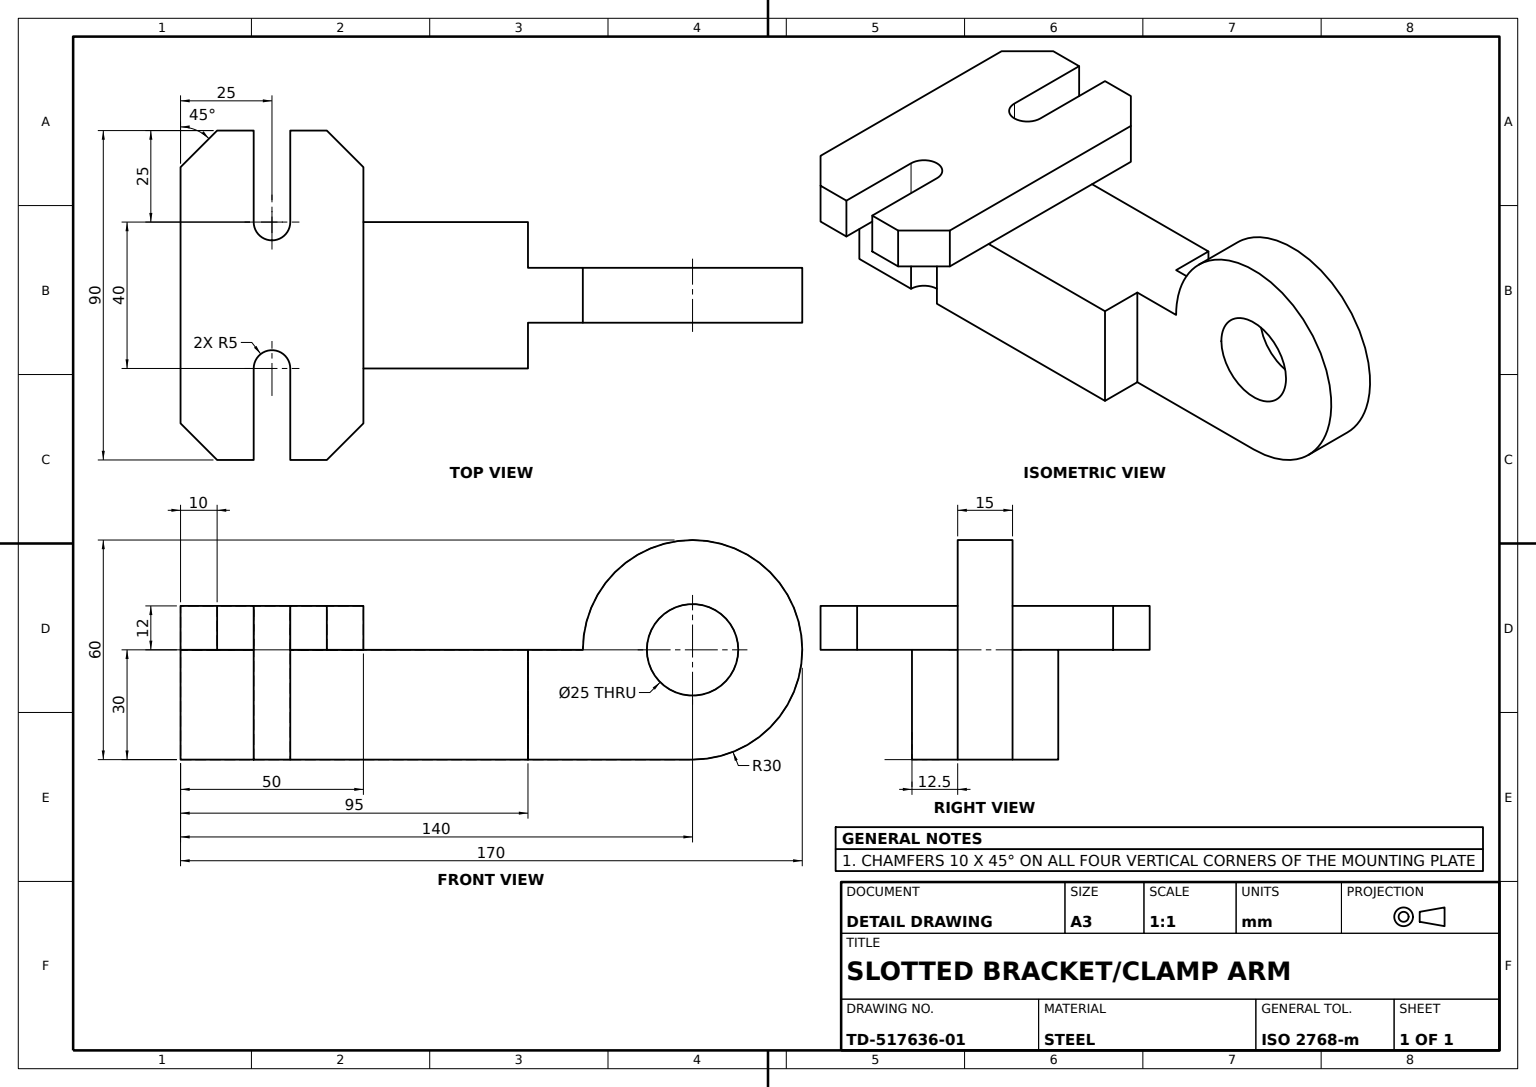
from build123d import *

# Parameters (mm, degrees)
ROD_BODY_SKETCH_W                = 95
ROD_BODY_SKETCH_H                = 30
ROD_BODY_30X95_DEPTH             = 20
MOUNTING_PLATE_SKETCH_W          = 50
MOUNTING_PLATE_SKETCH_H          = 90
MOUNTING_PLATE_12MM_DEPTH        = 12
EYE_BOSS_DEPTH                   = 7.5
EYE_HOLE_SKETCH_R                = 12.5
EYE_HOLE_25_DEPTH                = 15
MOUNTING_SLOTS_2X10_DEPTH        = 138.095769446
PLATE_CORNER_CHAMFERS_10X45_SIZE = 10


with BuildPart() as part:
    # Rod Body Sketch → Rod Body 30x95 (new, symmetric)
    with BuildSketch(Plane.XY):
        Rectangle(ROD_BODY_SKETCH_W, ROD_BODY_SKETCH_H)
    extrude(amount=ROD_BODY_30X95_DEPTH, both=True)

    # Mounting Plate Sketch → Mounting Plate 12mm (add)
    with BuildSketch(Plane(origin=(0, 15, 0), x_dir=(1, 0, 0), z_dir=(0, 1, 0))):
        with Locations((-22.5, 0)):
            Rectangle(MOUNTING_PLATE_SKETCH_W, MOUNTING_PLATE_SKETCH_H)
    extrude(amount=MOUNTING_PLATE_12MM_DEPTH)

    # Eye Boss Sketch → Eye Boss (add, symmetric)
    with BuildSketch(Plane.XY):
        with BuildLine():
            Line((92.5, -15), (47.5, -15))
            Line((47.5, -15), (47.5, 15))
            Line((47.5, 15), (62.5, 15))
            ThreePointArc((62.5, 15), (113.713203436, 36.213203436), (92.5, -15))
        make_face()
    extrude(amount=EYE_BOSS_DEPTH, both=True)

    # Eye Hole Sketch → Eye Hole Ø25 (cut)
    with BuildSketch(Plane.XY.offset(7.5)):
        with Locations((92.5, 15)):
            Circle(EYE_HOLE_SKETCH_R)
    extrude(amount=-EYE_HOLE_25_DEPTH, mode=Mode.SUBTRACT)

    # Mounting Slots Sketch → Mounting Slots 2x10 (cut, through all)
    with BuildSketch(Plane(origin=(0, 27, 0), x_dir=(1, 0, 0), z_dir=(0, 1, 0))):
        with BuildLine():
            Line((-27.5, 20), (-27.5, 45))
            Line((-27.5, 45), (-17.5, 45))
            Line((-17.5, 45), (-17.5, 20))
            ThreePointArc((-17.5, 20), (-22.5, 15), (-27.5, 20))
        make_face()
        with BuildLine():
            Line((-27.5, -20), (-27.5, -45))
            Line((-27.5, -45), (-17.5, -45))
            Line((-17.5, -45), (-17.5, -20))
            ThreePointArc((-17.5, -20), (-22.5, -15), (-27.5, -20))
        make_face()
    extrude(amount=-MOUNTING_SLOTS_2X10_DEPTH, mode=Mode.SUBTRACT)

    # Plate Corner Chamfers 10x45
    plate_corner_chamfers_10x45_edges = [part.edges().sort_by_distance(p)[0] for p in [
        (-47.5, 21, -45),
        (-47.5, 21, 45),
        (2.5, 21, 45),
        (2.5, 21, -45),
    ]]
    chamfer(plate_corner_chamfers_10x45_edges, length=PLATE_CORNER_CHAMFERS_10X45_SIZE)


solid = part.part
